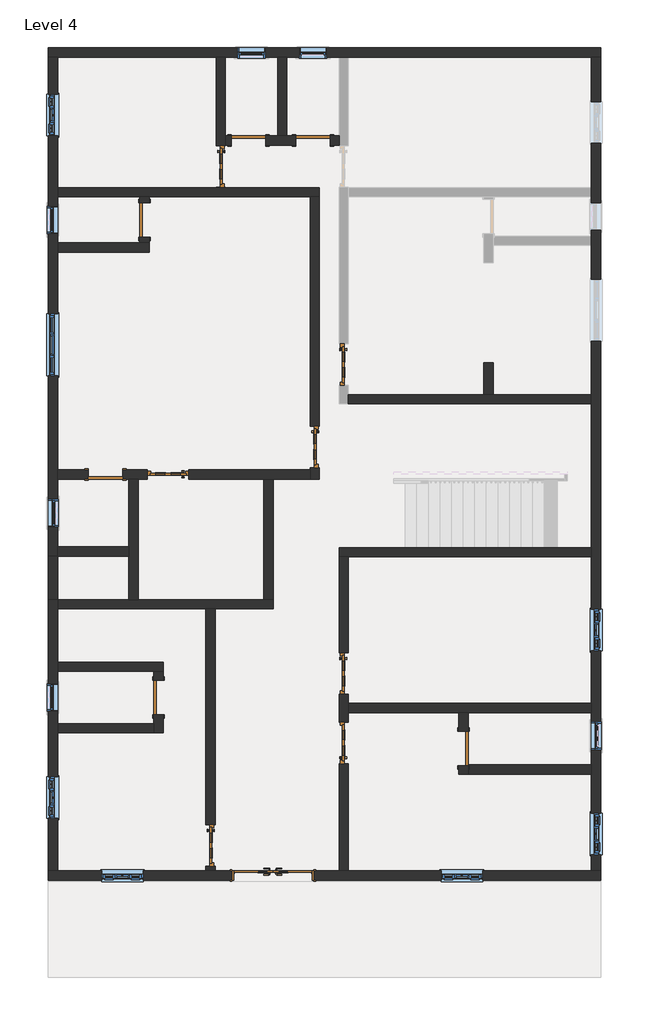
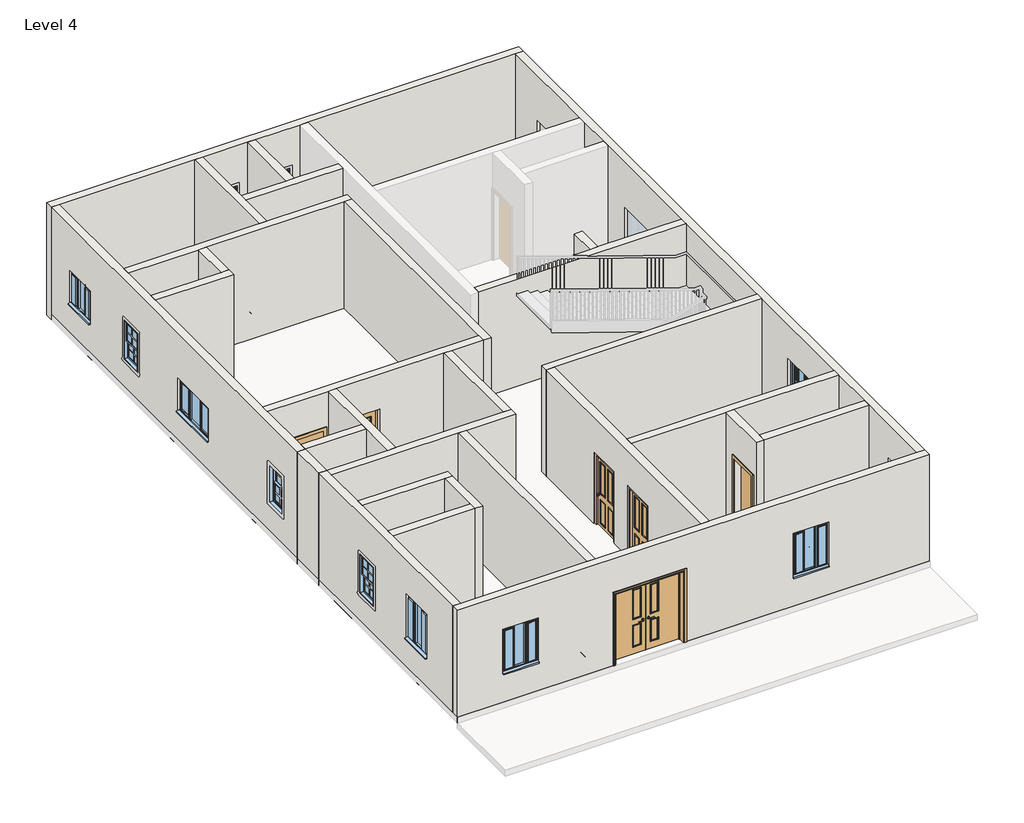
# One storey, part 1 of 3: 29 walls, 14 doors, 13 windows.
"""IFC4 building model written with IfcOpenShell, lengths in millimetres."""

from ifc_helpers import new_model, si_unit, frame, origin, place, context, project, spatial, polyline, outline, extrude, faceted_brep, transform, mapped, element, save
from components import door_2817e3e8, door_51b0c682, doors_intdbl_3_1810x2110mm_301b02ef, doors_intdbl_3_1810x2110mm_13513f6f, door_fadea3f2, door_53b1b562, window_679d2811, windows_tpl_plain_1360x910mm_84993ef1, windows_tpl_w_glazing_cross_bars_910x1210mm_e0b59135, windows_tpl_w_glazing_cross_bars_910x910mm_4aa0f884

model = new_model("IFC4")

# Units and contexts
model_context = context("Model", 3, world=origin())
ifc_project = project(units=[si_unit("LENGTHUNIT", "METRE", prefix="MILLI")], contexts=[model_context])

# Site, building, storey
site = spatial("IfcSite", under=ifc_project)
building = spatial("IfcBuilding", under=site)
storey = spatial("IfcBuildingStorey", under=building, Name="Level 4", Elevation=9144.0)

# Doors
placement = place(None, origin())
door_shape = door_2817e3e8(model_context)
element("IfcDoor", 1, ObjectType="Doors_ExtSgl_2 : 2'x7\"", at=placement, inside=storey, context=model_context, shape_type="MappedRepresentation", body=[
    mapped(door_shape, transform((-2349.4166288, 6357.8803322, 9144.0), x_axis=(0.0, -1.0, 0.0), y_axis=(1.0, 0.0, 0.0), z_axis=(0.0, 0.0, 1.0))),
])
element("IfcDoor", 2, ObjectType="Doors_ExtSgl_2 : 2'x7\"", at=placement, inside=storey, context=model_context, shape_type="MappedRepresentation", body=[
    mapped(door_shape, transform((-286.4451949, 208.0340986, 9144.0), x_axis=(0.0, -1.0, 0.0), y_axis=(1.0, 0.0, 0.0), z_axis=(0.0, 0.0, 1.0))),
])
element("IfcDoor", 3, ObjectType="Doors_ExtSgl_2 : 2'x7\"", at=placement, inside=storey, context=model_context, shape_type="MappedRepresentation", body=[
    mapped(door_shape, transform((348.5548051, -6285.6488489, 9144.0), x_axis=(0.0, 1.0, 0.0), y_axis=(-1.0, 0.0, 0.0), z_axis=(0.0, 0.0, 1.0))),
])
element("IfcDoor", 4, ObjectType="Doors_ExtSgl_2 : 2'x7\"", at=placement, inside=storey, context=model_context, shape_type="MappedRepresentation", body=[
    mapped(door_shape, transform((-2575.1220989, -8536.1734342, 9144.0), x_axis=(0.0, -1.0, 0.0), y_axis=(1.0, 0.0, 0.0), z_axis=(0.0, 0.0, 1.0))),
])
door_2_shape = door_51b0c682(model_context)
element("IfcDoor", 5, ObjectType="Doors_ExtSgl_2 : 2'x7\"", at=placement, inside=storey, context=model_context, shape_type="MappedRepresentation", body=[
    mapped(door_2_shape, transform((348.5548051, -4761.6488489, 9144.0), x_axis=(0.0, -1.0, 0.0), y_axis=(1.0, 0.0, 0.0), z_axis=(0.0, 0.0, 1.0))),
])
element("IfcDoor", 6, ObjectType="Doors_ExtSgl_2 : 2'x7\"", at=placement, inside=storey, context=model_context, shape_type="MappedRepresentation", body=[
    mapped(door_2_shape, transform((-3502.9153286, -401.5659014, 9144.0), x_axis=(-1.0, 0.0, 0.0), y_axis=(0.0, -1.0, 0.0), z_axis=(0.0, 0.0, 1.0))),
])
element("IfcDoor", 7, ObjectType="Doors_ExtSgl_2 : 2'x7\"", at=placement, inside=storey, context=model_context, shape_type="MappedRepresentation", body=[
    mapped(door_2_shape, transform((348.5548051, 2011.4340986, 9144.0), x_axis=(0.0, -1.0, 0.0), y_axis=(1.0, 0.0, 0.0), z_axis=(0.0, 0.0, 1.0))),
])
doors_intdbl_3_1810x2110mm_shape = doors_intdbl_3_1810x2110mm_301b02ef(model_context)
doors_intdbl_3_1810x2110mm_2_shape = doors_intdbl_3_1810x2110mm_13513f6f(model_context)
element("IfcDoor", 8, ObjectType="Doors_IntDbl_3 : 1810x2110mm", at=placement, inside=storey, context=model_context, shape_type="MappedRepresentation", body=[
    mapped(doors_intdbl_3_1810x2110mm_shape, transform((-1203.5220989, -9196.5734342, 9144.0), x_axis=(-1.0, 0.0, 0.0), y_axis=(0.0, -1.0, 0.0), z_axis=(0.0, 0.0, 1.0))),
    mapped(doors_intdbl_3_1810x2110mm_2_shape, transform((-1203.5220989, -9196.5734342, 9144.0), x_axis=(-1.0, 0.0, 0.0), y_axis=(0.0, -1.0, 0.0), z_axis=(0.0, 0.0, 1.0))),
])
door_3_shape = door_fadea3f2(model_context)
element("IfcDoor", 9, ObjectType="Single-Flush : 30\" x 80\"", at=placement, inside=storey, context=model_context, shape_type="MappedRepresentation", body=[
    mapped(door_3_shape, transform((-1739.8166288, 6926.3340986, 9144.0), x_axis=(1.0, 0.0, 0.0), y_axis=(0.0, 1.0, 0.0), z_axis=(0.0, 0.0, 1.0))),
])
element("IfcDoor", 10, ObjectType="Single-Flush : 30\" x 80\"", at=placement, inside=storey, context=model_context, shape_type="MappedRepresentation", body=[
    mapped(door_3_shape, transform((-4874.5153286, -401.5659014, 9144.0), x_axis=(-1.0, 0.0, 0.0), y_axis=(0.0, -1.0, 0.0), z_axis=(0.0, 0.0, 1.0))),
])
door_4_shape = door_53b1b562(model_context)
element("IfcDoor", 11, ObjectType="Single-Flush : 30\" x 80\"", at=placement, inside=storey, context=model_context, shape_type="MappedRepresentation", body=[
    mapped(door_4_shape, transform((-324.5451949, 6926.3340986, 9144.0), x_axis=(-1.0, 0.0, 0.0), y_axis=(0.0, -1.0, 0.0), z_axis=(0.0, 0.0, 1.0))),
])
element("IfcDoor", 12, ObjectType="Single-Flush : 30\" x 80\"", at=placement, inside=storey, context=model_context, shape_type="MappedRepresentation", body=[
    mapped(door_4_shape, transform((-3715.4451949, -5291.0659014, 9144.0), x_axis=(0.0, -1.0, 0.0), y_axis=(1.0, 0.0, 0.0), z_axis=(0.0, 0.0, 1.0))),
])
element("IfcDoor", 13, ObjectType="Single-Flush : 30\" x 80\"", at=placement, inside=storey, context=model_context, shape_type="MappedRepresentation", body=[
    mapped(door_4_shape, transform((2977.4548051, -6412.6488489, 9144.0), x_axis=(0.0, 1.0, 0.0), y_axis=(-1.0, 0.0, 0.0), z_axis=(0.0, 0.0, 1.0))),
])
element("IfcDoor", 14, ObjectType="Single-Flush : 30\" x 80\"", at=placement, inside=storey, context=model_context, shape_type="MappedRepresentation", body=[
    mapped(door_4_shape, transform((-4023.5839448, 5183.1303322, 9144.0), x_axis=(0.0, -1.0, 0.0), y_axis=(1.0, 0.0, 0.0), z_axis=(0.0, 0.0, 1.0))),
])

# Walls
element("IfcWall", 15, ObjectType="Generic - 4.5\" p", at=placement, inside=storey, context=model_context, shape_type="Brep", body=[
    faceted_brep([(-5928.5839448, 5687.8265658, 9144.0), (-4125.1839448, 5687.8265658, 9144.0), (-3921.9839448, 5687.8265658, 9144.0), (-388.0451949, 5687.8265658, 9144.0), (-184.8451949, 5687.8265658, 9144.0), (-184.8451949, 5687.8265658, 12192.0), (-388.0451949, 5687.8265658, 12192.0), (-3921.9839448, 5687.8265658, 12192.0), (-4125.1839448, 5687.8265658, 12192.0), (-5928.5839448, 5687.8265658, 12192.0), (-5928.5839448, 5891.0265658, 9144.0), (-5928.5839448, 5891.0265658, 12192.0), (-2451.0166288, 5891.0265658, 12192.0), (-2247.8166288, 5891.0265658, 12192.0), (-184.8451949, 5891.0265658, 12192.0), (-184.8451949, 5891.0265658, 9144.0), (-2247.8166288, 5891.0265658, 9144.0), (-2451.0166288, 5891.0265658, 9144.0)], [[[0, 1, 2, 3, 4, 5, 6, 7, 8, 9]], [[10, 11, 12, 13, 14, 15, 16, 17]], [[4, 3, 2, 1, 0, 10, 17, 16, 15]], [[0, 9, 11, 10]], [[5, 4, 15, 14]], [[9, 8, 7, 6, 5, 14, 13, 12, 11]]]),
])
element("IfcWall", 16, ObjectType="Generic - 4.5\" p", at=placement, inside=storey, context=model_context, shape_type="Brep", body=[
    faceted_brep([(-388.0451949, -246.9659014, 11254.0), (-388.0451949, -246.9659014, 9144.0), (-388.0451949, -299.9659014, 9144.0), (-388.0451949, -503.1659014, 9144.0), (-388.0451949, -503.1659014, 12192.0), (-388.0451949, -299.9659014, 12192.0), (-388.0451949, 5687.8265658, 12192.0), (-388.0451949, 5687.8265658, 9144.0), (-388.0451949, 663.0340986, 9144.0), (-388.0451949, 663.0340986, 11254.0), (-184.8451949, -503.1659014, 9144.0), (-184.8451949, -246.9659014, 9144.0), (-184.8451949, -246.9659014, 11254.0), (-184.8451949, 663.0340986, 11254.0), (-184.8451949, 663.0340986, 9144.0), (-184.8451949, 5687.8265658, 9144.0), (-184.8451949, 5687.8265658, 12192.0), (-184.8451949, -503.1659014, 12192.0)], [[[0, 1, 2, 3, 4, 5, 6, 7, 8, 9]], [[10, 11, 12, 13, 14, 15, 16, 17]], [[8, 7, 15, 14]], [[3, 2, 1, 11, 10]], [[7, 6, 16, 15]], [[4, 3, 10, 17]], [[14, 13, 9, 8]], [[12, 11, 1, 0]], [[13, 12, 0, 9]], [[6, 5, 4, 17, 16]]]),
])
element("IfcWall", 17, ObjectType="Generic - 4.5\" p", at=placement, inside=storey, context=model_context, shape_type="Brep", body=[
    faceted_brep([(-5255.5153286, -299.9659014, 11176.0), (-5255.5153286, -299.9659014, 9144.0), (-5928.5839448, -299.9659014, 9144.0), (-5928.5839448, -299.9659014, 12192.0), (-388.0451949, -299.9659014, 12192.0), (-388.0451949, -299.9659014, 9144.0), (-3047.9153286, -299.9659014, 9144.0), (-3047.9153286, -299.9659014, 11254.0), (-3957.9153286, -299.9659014, 11254.0), (-3957.9153286, -299.9659014, 9144.0), (-4493.5153286, -299.9659014, 9144.0), (-4493.5153286, -299.9659014, 11176.0), (-5928.5839448, -503.1659014, 9144.0), (-5255.5153286, -503.1659014, 9144.0), (-5255.5153286, -503.1659014, 11176.0), (-4493.5153286, -503.1659014, 11176.0), (-4493.5153286, -503.1659014, 9144.0), (-4366.5153286, -503.1659014, 9144.0), (-4163.3153286, -503.1659014, 9144.0), (-3957.9153286, -503.1659014, 9144.0), (-3957.9153286, -503.1659014, 11254.0), (-3047.9153286, -503.1659014, 11254.0), (-3047.9153286, -503.1659014, 9144.0), (-1404.0451949, -503.1659014, 9144.0), (-1200.8451949, -503.1659014, 9144.0), (-388.0451949, -503.1659014, 9144.0), (-388.0451949, -503.1659014, 12192.0), (-1200.8451949, -503.1659014, 12192.0), (-1404.0451949, -503.1659014, 12192.0), (-4163.3153286, -503.1659014, 12192.0), (-4366.5153286, -503.1659014, 12192.0), (-5928.5839448, -503.1659014, 12192.0)], [[[0, 1, 2, 3, 4, 5, 6, 7, 8, 9, 10, 11]], [[12, 13, 14, 15, 16, 17, 18, 19, 20, 21, 22, 23, 24, 25, 26, 27, 28, 29, 30, 31]], [[6, 5, 25, 24, 23, 22]], [[10, 9, 19, 18, 17, 16]], [[2, 1, 13, 12]], [[5, 4, 26, 25]], [[3, 2, 12, 31]], [[22, 21, 7, 6]], [[20, 19, 9, 8]], [[21, 20, 8, 7]], [[14, 13, 1, 0]], [[15, 14, 0, 11]], [[16, 15, 11, 10]], [[4, 3, 31, 30, 29, 28, 27, 26]]]),
])
element("IfcWall", 18, ObjectType="Generic - 4.5\" p", at=placement, inside=storey, context=model_context, shape_type="Brep", body=[
    faceted_brep([(-4366.5153286, -503.1659014, 9144.0), (-4366.5153286, -1989.0659014, 9144.0), (-4366.5153286, -2192.2659014, 9144.0), (-4366.5153286, -3144.7659014, 9144.0), (-4366.5153286, -3144.7659014, 12192.0), (-4366.5153286, -2192.2659014, 12192.0), (-4366.5153286, -1989.0659014, 12192.0), (-4366.5153286, -503.1659014, 12192.0), (-4163.3153286, -503.1659014, 9144.0), (-4163.3153286, -503.1659014, 12192.0), (-4163.3153286, -3144.7659014, 12192.0), (-4163.3153286, -3144.7659014, 9144.0)], [[[0, 1, 2, 3, 4, 5, 6, 7]], [[8, 9, 10, 11]], [[3, 2, 1, 0, 8, 11]], [[0, 7, 9, 8]], [[4, 3, 11, 10]], [[7, 6, 5, 4, 10, 9]]]),
])
element("IfcWall", 19, ObjectType="Generic - 4.5\" p", at=placement, inside=storey, context=model_context, shape_type="Brep", body=[
    faceted_brep([(-5928.5839448, -3347.9659014, 9144.0), (-2676.7220989, -3347.9659014, 9144.0), (-2473.5220989, -3347.9659014, 9144.0), (-1200.8451949, -3347.9659014, 9144.0), (-1200.8451949, -3347.9659014, 12192.0), (-2473.5220989, -3347.9659014, 12192.0), (-2676.7220989, -3347.9659014, 12192.0), (-5928.5839448, -3347.9659014, 12192.0), (-5928.5839448, -3144.7659014, 9144.0), (-5928.5839448, -3144.7659014, 12192.0), (-4366.5153286, -3144.7659014, 12192.0), (-4163.3153286, -3144.7659014, 12192.0), (-1404.0451949, -3144.7659014, 12192.0), (-1200.8451949, -3144.7659014, 12192.0), (-1200.8451949, -3144.7659014, 9144.0), (-1404.0451949, -3144.7659014, 9144.0), (-4163.3153286, -3144.7659014, 9144.0), (-4366.5153286, -3144.7659014, 9144.0)], [[[0, 1, 2, 3, 4, 5, 6, 7]], [[8, 9, 10, 11, 12, 13, 14, 15, 16, 17]], [[3, 2, 1, 0, 8, 17, 16, 15, 14]], [[0, 7, 9, 8]], [[4, 3, 14, 13]], [[7, 6, 5, 4, 13, 12, 11, 10, 9]]]),
])
element("IfcWall", 20, ObjectType="Generic - 4.5\" p", at=placement, inside=storey, context=model_context, shape_type="SweptSolid", body=[
    extrude(outline(polyline([(-4366.5153286, -2192.2659014), (-5928.5839448, -2192.2659014), (-5928.5839448, -1989.0659014), (-4366.5153286, -1989.0659014), (-4366.5153286, -2192.2659014)])), frame((0.0, 0.0, 9144.0), z_axis=(0.0, 0.0, 1.0), x_axis=(1.0, 0.0, 0.0)), (0.0, 0.0, 1.0), 3048.0),
])
element("IfcWall", 21, ObjectType="Generic - 4.5\" p", at=placement, inside=storey, context=model_context, shape_type="SweptSolid", body=[
    extrude(outline(polyline([(-1404.0451949, -3144.7659014), (-1404.0451949, -503.1659014), (-1200.8451949, -503.1659014), (-1200.8451949, -3144.7659014), (-1404.0451949, -3144.7659014)])), frame((0.0, 0.0, 9144.0), z_axis=(0.0, 0.0, 1.0), x_axis=(1.0, 0.0, 0.0)), (0.0, 0.0, 1.0), 3048.0),
])
element("IfcWall", 22, ObjectType="Generic - 4.5\" p", at=placement, inside=storey, context=model_context, shape_type="Brep", body=[
    faceted_brep([(-5928.5839448, -4719.5659014, 9144.0), (-3817.0451949, -4719.5659014, 9144.0), (-3613.8451949, -4719.5659014, 9144.0), (-3613.8451949, -4719.5659014, 12192.0), (-3817.0451949, -4719.5659014, 12192.0), (-5928.5839448, -4719.5659014, 12192.0), (-5928.5839448, -4516.3659014, 9144.0), (-5928.5839448, -4516.3659014, 12192.0), (-3613.8451949, -4516.3659014, 12192.0), (-3613.8451949, -4516.3659014, 9144.0)], [[[0, 1, 2, 3, 4, 5]], [[6, 7, 8, 9]], [[2, 1, 0, 6, 9]], [[0, 5, 7, 6]], [[3, 2, 9, 8]], [[5, 4, 3, 8, 7]]]),
])
element("IfcWall", 23, ObjectType="Generic - 4.5\" p", at=placement, inside=storey, context=model_context, shape_type="Brep", body=[
    faceted_brep([(-3817.0451949, -5672.0659014, 11176.0), (-3817.0451949, -5672.0659014, 9144.0), (-3817.0451949, -5862.5659014, 9144.0), (-3817.0451949, -6065.7659014, 9144.0), (-3817.0451949, -6065.7659014, 12192.0), (-3817.0451949, -5862.5659014, 12192.0), (-3817.0451949, -4719.5659014, 12192.0), (-3817.0451949, -4719.5659014, 9144.0), (-3817.0451949, -4910.0659014, 9144.0), (-3817.0451949, -4910.0659014, 11176.0), (-3613.8451949, -6065.7659014, 9144.0), (-3613.8451949, -5672.0659014, 9144.0), (-3613.8451949, -5672.0659014, 11176.0), (-3613.8451949, -4910.0659014, 11176.0), (-3613.8451949, -4910.0659014, 9144.0), (-3613.8451949, -4719.5659014, 9144.0), (-3613.8451949, -4719.5659014, 12192.0), (-3613.8451949, -6065.7659014, 12192.0)], [[[0, 1, 2, 3, 4, 5, 6, 7, 8, 9]], [[10, 11, 12, 13, 14, 15, 16, 17]], [[8, 7, 15, 14]], [[3, 2, 1, 11, 10]], [[7, 6, 16, 15]], [[4, 3, 10, 17]], [[12, 11, 1, 0]], [[13, 12, 0, 9]], [[14, 13, 9, 8]], [[6, 5, 4, 17, 16]]]),
])
element("IfcWall", 24, ObjectType="Generic - 4.5\" p", at=placement, inside=storey, context=model_context, shape_type="SweptSolid", body=[
    extrude(outline(polyline([(-5928.5839448, -5862.5659014), (-3817.0451949, -5862.5659014), (-3817.0451949, -6065.7659014), (-5928.5839448, -6065.7659014), (-5928.5839448, -5862.5659014)])), frame((0.0, 0.0, 9144.0), z_axis=(0.0, 0.0, 1.0), x_axis=(1.0, 0.0, 0.0)), (0.0, 0.0, 1.0), 3048.0),
])
element("IfcWall", 25, ObjectType="Generic - 4.5\" p", at=placement, inside=storey, context=model_context, shape_type="SweptSolid", body=[
    extrude(outline(polyline([(-8991.1734342, 11254.0), (-8991.1734342, 9144.0), (-9094.9734342, 9144.0), (-9094.9734342, 12192.0), (-3347.9659014, 12192.0), (-3347.9659014, 9144.0), (-8081.1734342, 9144.0), (-8081.1734342, 11254.0), (-8991.1734342, 11254.0)])), frame((-2676.7220989, 0.0, 0.0), z_axis=(1.0, 0.0, 0.0), x_axis=(0.0, 1.0, 0.0)), (0.0, 0.0, 1.0), 203.2),
])
element("IfcWall", 26, ObjectType="Generic - 4.5\" p", at=placement, inside=storey, context=model_context, shape_type="Brep", body=[
    faceted_brep([(-5928.5839448, 4475.2340986, 9144.0), (-3921.9839448, 4475.2340986, 9144.0), (-3921.9839448, 4475.2340986, 12192.0), (-5928.5839448, 4475.2340986, 12192.0), (-5928.5839448, 4678.4340986, 9144.0), (-5928.5839448, 4678.4340986, 12192.0), (-4125.1839448, 4678.4340986, 12192.0), (-3921.9839448, 4678.4340986, 12192.0), (-3921.9839448, 4678.4340986, 9144.0), (-4125.1839448, 4678.4340986, 9144.0)], [[[0, 1, 2, 3]], [[4, 5, 6, 7, 8, 9]], [[1, 0, 4, 9, 8]], [[0, 3, 5, 4]], [[2, 1, 8, 7]], [[3, 2, 7, 6, 5]]]),
])
element("IfcWall", 27, ObjectType="Generic - 4.5\" p", at=placement, inside=storey, context=model_context, shape_type="SweptSolid", body=[
    extrude(outline(polyline([(4802.1303322, 11176.0), (4802.1303322, 9144.0), (4678.4340986, 9144.0), (4678.4340986, 12192.0), (5687.8265658, 12192.0), (5687.8265658, 9144.0), (5564.1303322, 9144.0), (5564.1303322, 11176.0), (4802.1303322, 11176.0)])), frame((-4125.1839448, 0.0, 0.0), z_axis=(1.0, 0.0, 0.0), x_axis=(0.0, 1.0, 0.0)), (0.0, 0.0, 1.0), 203.2),
])
element("IfcWall", 28, ObjectType="Generic - 4.5\" p", at=placement, inside=storey, context=model_context, shape_type="Brep", body=[
    faceted_brep([(-2451.0166288, 5902.8803322, 11254.0), (-2451.0166288, 5902.8803322, 9144.0), (-2451.0166288, 5891.0265658, 9144.0), (-2451.0166288, 5891.0265658, 12192.0), (-2451.0166288, 8752.5974079, 12192.0), (-2451.0166288, 8752.5974079, 9144.0), (-2451.0166288, 6812.8803322, 9144.0), (-2451.0166288, 6812.8803322, 11254.0), (-2247.8166288, 5891.0265658, 9144.0), (-2247.8166288, 5902.8803322, 9144.0), (-2247.8166288, 5902.8803322, 11254.0), (-2247.8166288, 6812.8803322, 11254.0), (-2247.8166288, 6812.8803322, 9144.0), (-2247.8166288, 6824.7340986, 9144.0), (-2247.8166288, 7027.9340986, 9144.0), (-2247.8166288, 8752.5974079, 9144.0), (-2247.8166288, 8752.5974079, 12192.0), (-2247.8166288, 7027.9340986, 12192.0), (-2247.8166288, 6824.7340986, 12192.0), (-2247.8166288, 5891.0265658, 12192.0)], [[[0, 1, 2, 3, 4, 5, 6, 7]], [[8, 9, 10, 11, 12, 13, 14, 15, 16, 17, 18, 19]], [[6, 5, 15, 14, 13, 12]], [[2, 1, 9, 8]], [[5, 4, 16, 15]], [[3, 2, 8, 19]], [[12, 11, 7, 6]], [[10, 9, 1, 0]], [[11, 10, 0, 7]], [[4, 3, 19, 18, 17, 16]]]),
])
element("IfcWall", 29, ObjectType="Generic - 4.5\" p", at=placement, inside=storey, context=model_context, shape_type="Brep", body=[
    faceted_brep([(-1358.8166288, 6824.7340986, 9144.0), (-705.5451949, 6824.7340986, 9144.0), (-705.5451949, 6824.7340986, 11176.0), (56.4548051, 6824.7340986, 11176.0), (56.4548051, 6824.7340986, 9144.0), (246.9548051, 6824.7340986, 9144.0), (246.9548051, 6824.7340986, 12192.0), (-2247.8166288, 6824.7340986, 12192.0), (-2247.8166288, 6824.7340986, 9144.0), (-2120.8166288, 6824.7340986, 9144.0), (-2120.8166288, 6824.7340986, 11176.0), (-1358.8166288, 6824.7340986, 11176.0), (-705.5451949, 7027.9340986, 11176.0), (-705.5451949, 7027.9340986, 9144.0), (-896.0451949, 7027.9340986, 9144.0), (-1099.2451949, 7027.9340986, 9144.0), (-1358.8166288, 7027.9340986, 9144.0), (-1358.8166288, 7027.9340986, 11176.0), (-2120.8166288, 7027.9340986, 11176.0), (-2120.8166288, 7027.9340986, 9144.0), (-2247.8166288, 7027.9340986, 9144.0), (-2247.8166288, 7027.9340986, 12192.0), (-1099.2451949, 7027.9340986, 12192.0), (-896.0451949, 7027.9340986, 12192.0), (246.9548051, 7027.9340986, 12192.0), (246.9548051, 7027.9340986, 9144.0), (56.4548051, 7027.9340986, 9144.0), (56.4548051, 7027.9340986, 11176.0)], [[[0, 1, 2, 3, 4, 5, 6, 7, 8, 9, 10, 11]], [[12, 13, 14, 15, 16, 17, 18, 19, 20, 21, 22, 23, 24, 25, 26, 27]], [[9, 8, 20, 19]], [[26, 25, 5, 4]], [[16, 15, 14, 13, 1, 0]], [[8, 7, 21, 20]], [[6, 5, 25, 24]], [[17, 16, 0, 11]], [[18, 17, 11, 10]], [[19, 18, 10, 9]], [[2, 1, 13, 12]], [[3, 2, 12, 27]], [[4, 3, 27, 26]], [[7, 6, 24, 23, 22, 21]]]),
])
element("IfcWall", 30, ObjectType="Generic - 4.5\" p", at=placement, inside=storey, context=model_context, shape_type="SweptSolid", body=[
    extrude(outline(polyline([(-1099.2451949, 7027.9340986), (-1099.2451949, 8752.5974079), (-896.0451949, 8752.5974079), (-896.0451949, 7027.9340986), (-1099.2451949, 7027.9340986)])), frame((0.0, 0.0, 9144.0), z_axis=(0.0, 0.0, 1.0), x_axis=(1.0, 0.0, 0.0)), (0.0, 0.0, 1.0), 3048.0),
])
element("IfcWall", 31, ObjectType="Generic - 4.5\" p", at=placement, inside=storey, context=model_context, shape_type="Brep", body=[
    faceted_brep([(450.1548051, 1147.8340986, 9144.0), (5778.5439795, 1147.8340986, 9144.0), (5778.5439795, 1147.8340986, 12192.0), (450.1548051, 1147.8340986, 12192.0), (450.1548051, 1351.0340986, 9144.0), (450.1548051, 1351.0340986, 12192.0), (3421.9548051, 1351.0340986, 12192.0), (3625.1548051, 1351.0340986, 12192.0), (5778.5439795, 1351.0340986, 12192.0), (5778.5439795, 1351.0340986, 9144.0), (3625.1548051, 1351.0340986, 9144.0), (3421.9548051, 1351.0340986, 9144.0)], [[[0, 1, 2, 3]], [[4, 5, 6, 7, 8, 9, 10, 11]], [[1, 0, 4, 11, 10, 9]], [[0, 3, 5, 4]], [[2, 1, 9, 8]], [[3, 2, 8, 7, 6, 5]]]),
])
element("IfcWall", 32, ObjectType="Generic - 4.5\" p", at=placement, inside=storey, context=model_context, shape_type="SweptSolid", body=[
    extrude(outline(polyline([(3625.1548051, 2047.4361958), (3625.1548051, 1351.0340986), (3421.9548051, 1351.0340986), (3421.9548051, 2047.4361958), (3625.1548051, 2047.4361958)])), frame((0.0, 0.0, 9144.0), z_axis=(0.0, 0.0, 1.0), x_axis=(1.0, 0.0, 0.0)), (0.0, 0.0, 1.0), 3048.0),
])
element("IfcWall", 33, ObjectType="Generic - 4.5\" p", at=placement, inside=storey, context=model_context, shape_type="Brep", body=[
    faceted_brep([(5778.5439795, -2004.8977001, 9144.0), (246.9548051, -2004.8977001, 9144.0), (246.9548051, -2004.8977001, 12192.0), (5778.5439795, -2004.8977001, 12192.0), (5778.5439795, -2208.0977001, 9144.0), (5778.5439795, -2208.0977001, 12192.0), (450.1548051, -2208.0977001, 12192.0), (246.9548051, -2208.0977001, 12192.0), (246.9548051, -2208.0977001, 9144.0), (450.1548051, -2208.0977001, 9144.0)], [[[0, 1, 2, 3]], [[4, 5, 6, 7, 8, 9]], [[1, 0, 4, 9, 8]], [[0, 3, 5, 4]], [[2, 1, 8, 7]], [[3, 2, 7, 6, 5]]]),
])
element("IfcWall", 34, ObjectType="Generic - 4.5\" p", at=placement, inside=storey, context=model_context, shape_type="Brep", body=[
    faceted_brep([(246.9548051, -5216.6488489, 9144.0), (246.9548051, -5830.6488489, 9144.0), (246.9548051, -5830.6488489, 11254.0), (246.9548051, -6740.6488489, 11254.0), (246.9548051, -6740.6488489, 9144.0), (246.9548051, -9094.9734342, 9144.0), (246.9548051, -9094.9734342, 12192.0), (246.9548051, -2208.0977001, 12192.0), (246.9548051, -2208.0977001, 9144.0), (246.9548051, -4306.6488489, 9144.0), (246.9548051, -4306.6488489, 11254.0), (246.9548051, -5216.6488489, 11254.0), (450.1548051, -5830.6488489, 11254.0), (450.1548051, -5830.6488489, 9144.0), (450.1548051, -5625.2488489, 9144.0), (450.1548051, -5422.0488489, 9144.0), (450.1548051, -5216.6488489, 9144.0), (450.1548051, -5216.6488489, 11254.0), (450.1548051, -4306.6488489, 11254.0), (450.1548051, -4306.6488489, 9144.0), (450.1548051, -2208.0977001, 9144.0), (450.1548051, -2208.0977001, 12192.0), (450.1548051, -5422.0488489, 12192.0), (450.1548051, -5625.2488489, 12192.0), (450.1548051, -9094.9734342, 12192.0), (450.1548051, -9094.9734342, 9144.0), (450.1548051, -6740.6488489, 9144.0), (450.1548051, -6740.6488489, 11254.0)], [[[0, 1, 2, 3, 4, 5, 6, 7, 8, 9, 10, 11]], [[12, 13, 14, 15, 16, 17, 18, 19, 20, 21, 22, 23, 24, 25, 26, 27]], [[9, 8, 20, 19]], [[26, 25, 5, 4]], [[16, 15, 14, 13, 1, 0]], [[8, 7, 21, 20]], [[6, 5, 25, 24]], [[19, 18, 10, 9]], [[17, 16, 0, 11]], [[18, 17, 11, 10]], [[4, 3, 27, 26]], [[2, 1, 13, 12]], [[3, 2, 12, 27]], [[7, 6, 24, 23, 22, 21]]]),
])
element("IfcWall", 35, ObjectType="Generic - 4.5\" p", at=placement, inside=storey, context=model_context, shape_type="Brep", body=[
    faceted_brep([(450.1548051, -5625.2488489, 9144.0), (2875.8548051, -5625.2488489, 9144.0), (3079.0548051, -5625.2488489, 9144.0), (5778.5439795, -5625.2488489, 9144.0), (5778.5439795, -5625.2488489, 12192.0), (3079.0548051, -5625.2488489, 12192.0), (2875.8548051, -5625.2488489, 12192.0), (450.1548051, -5625.2488489, 12192.0), (450.1548051, -5422.0488489, 9144.0), (450.1548051, -5422.0488489, 12192.0), (5778.5439795, -5422.0488489, 12192.0), (5778.5439795, -5422.0488489, 9144.0)], [[[0, 1, 2, 3, 4, 5, 6, 7]], [[8, 9, 10, 11]], [[3, 2, 1, 0, 8, 11]], [[4, 3, 11, 10]], [[0, 7, 9, 8]], [[7, 6, 5, 4, 10, 9]]]),
])
element("IfcWall", 36, ObjectType="Generic - 4.5\" p", at=placement, inside=storey, context=model_context, shape_type="Brep", body=[
    faceted_brep([(2875.8548051, -5625.2488489, 9144.0), (2875.8548051, -6031.6488489, 9144.0), (2875.8548051, -6031.6488489, 11176.0), (2875.8548051, -6793.6488489, 11176.0), (2875.8548051, -6793.6488489, 9144.0), (2875.8548051, -6971.4488489, 9144.0), (2875.8548051, -6971.4488489, 12192.0), (2875.8548051, -5625.2488489, 12192.0), (3079.0548051, -6031.6488489, 11176.0), (3079.0548051, -6031.6488489, 9144.0), (3079.0548051, -5625.2488489, 9144.0), (3079.0548051, -5625.2488489, 12192.0), (3079.0548051, -6768.2488489, 12192.0), (3079.0548051, -6971.4488489, 12192.0), (3079.0548051, -6971.4488489, 9144.0), (3079.0548051, -6793.6488489, 9144.0), (3079.0548051, -6793.6488489, 11176.0)], [[[0, 1, 2, 3, 4, 5, 6, 7]], [[8, 9, 10, 11, 12, 13, 14, 15, 16]], [[10, 9, 1, 0]], [[15, 14, 5, 4]], [[0, 7, 11, 10]], [[6, 5, 14, 13]], [[2, 1, 9, 8]], [[3, 2, 8, 16]], [[4, 3, 16, 15]], [[7, 6, 13, 12, 11]]]),
])
element("IfcWall", 37, ObjectType="Generic - 4.5\" p", at=placement, inside=storey, context=model_context, shape_type="Brep", body=[
    faceted_brep([(5778.5439795, -6768.2488489, 9144.0), (3079.0548051, -6768.2488489, 9144.0), (3079.0548051, -6768.2488489, 12192.0), (5778.5439795, -6768.2488489, 12192.0), (5778.5439795, -6971.4488489, 9144.0), (5778.5439795, -6971.4488489, 12192.0), (3079.0548051, -6971.4488489, 12192.0), (3079.0548051, -6971.4488489, 9144.0), (3079.0548051, -6793.6488489, 9144.0)], [[[0, 1, 2, 3]], [[4, 5, 6, 7]], [[1, 0, 4, 7, 8]], [[2, 1, 8, 7, 6]], [[0, 3, 5, 4]], [[3, 2, 6, 5]]]),
])
element("IfcWall", 38, ObjectType="Generic - 4.5\" p", at=placement, inside=storey, context=model_context, shape_type="SweptSolid", body=[
    extrude(outline(polyline([(-6131.7839448, -3144.7659014), (-6131.7839448, -2192.2659014), (-5928.5839448, -2192.2659014), (-5928.5839448, -3144.7659014), (-6131.7839448, -3144.7659014)])), frame((0.0, 0.0, 9144.0), z_axis=(0.0, 0.0, 1.0), x_axis=(1.0, 0.0, 0.0)), (0.0, 0.0, 1.0), 3048.0),
])
element("IfcWall", 39, ObjectType="Generic - 9\" w", at=placement, inside=storey, context=model_context, shape_type="Brep", body=[
    faceted_brep([(-6134.0560205, 8752.5974079, 9144.0), (-6131.7839448, 8752.5974079, 9144.0), (-5928.5839448, 8752.5974079, 9144.0), (-2451.0166288, 8752.5974079, 9144.0), (-2247.8166288, 8752.5974079, 9144.0), (-1099.2451949, 8752.5974079, 9144.0), (-896.0451949, 8752.5974079, 9144.0), (246.9548051, 8752.5974079, 9144.0), (450.1548051, 8752.5974079, 9144.0), (5778.5439795, 8752.5974079, 9144.0), (5981.7439795, 8752.5974079, 9144.0), (5981.7439795, 8752.5974079, 12192.0), (5778.5439795, 8752.5974079, 12192.0), (450.1548051, 8752.5974079, 12192.0), (246.9548051, 8752.5974079, 12192.0), (-896.0451949, 8752.5974079, 12192.0), (-1099.2451949, 8752.5974079, 12192.0), (-2247.8166288, 8752.5974079, 12192.0), (-2451.0166288, 8752.5974079, 12192.0), (-5928.5839448, 8752.5974079, 12192.0), (-6131.7839448, 8752.5974079, 12192.0), (-6134.0560205, 8752.5974079, 12192.0), (-1368.7309118, 8752.5974079, 11125.2), (-1368.7309118, 8752.5974079, 10058.4), (-1978.3309118, 8752.5974079, 10058.4), (-1978.3309118, 8752.5974079, 11125.2), (-19.7451949, 8752.5974079, 11125.2), (-19.7451949, 8752.5974079, 10058.4), (-629.3451949, 8752.5974079, 10058.4), (-629.3451949, 8752.5974079, 11125.2), (-6134.0560205, 8955.7974079, 9144.0), (-6134.0560205, 8955.7974079, 12192.0), (5981.7439795, 8955.7974079, 12192.0), (5981.7439795, 8955.7974079, 9144.0), (-1368.7309118, 8955.7974079, 11125.2), (-1978.3309118, 8955.7974079, 11125.2), (-1978.3309118, 8955.7974079, 10058.4), (-1368.7309118, 8955.7974079, 10058.4), (-19.7451949, 8955.7974079, 11125.2), (-629.3451949, 8955.7974079, 11125.2), (-629.3451949, 8955.7974079, 10058.4), (-19.7451949, 8955.7974079, 10058.4)], [[[0, 1, 2, 3, 4, 5, 6, 7, 8, 9, 10, 11, 12, 13, 14, 15, 16, 17, 18, 19, 20, 21], [22, 23, 24, 25], [26, 27, 28, 29]], [[30, 31, 32, 33], [34, 35, 36, 37], [38, 39, 40, 41]], [[10, 9, 8, 7, 6, 5, 4, 3, 2, 1, 0, 30, 33]], [[0, 21, 31, 30]], [[11, 10, 33, 32]], [[23, 22, 34, 37]], [[24, 23, 37, 36]], [[25, 24, 36, 35]], [[22, 25, 35, 34]], [[27, 26, 38, 41]], [[28, 27, 41, 40]], [[29, 28, 40, 39]], [[26, 29, 39, 38]], [[21, 20, 19, 18, 17, 16, 15, 14, 13, 12, 11, 32, 31]]]),
])
element("IfcWall", 40, ObjectType="Generic - 9\" w", at=placement, inside=storey, context=model_context, shape_type="Brep", body=[
    faceted_brep([(5981.7439795, -9094.9734342, 12192.0), (5981.7439795, -9094.9734342, 9144.0), (5778.5439795, -9094.9734342, 9144.0), (450.1548051, -9094.9734342, 9144.0), (246.9548051, -9094.9734342, 9144.0), (-298.5220989, -9094.9734342, 9144.0), (-298.5220989, -9094.9734342, 11254.0), (-2108.5220989, -9094.9734342, 11254.0), (-2108.5220989, -9094.9734342, 9144.0), (-2473.5220989, -9094.9734342, 9144.0), (-2676.7220989, -9094.9734342, 9144.0), (-5928.5839448, -9094.9734342, 9144.0), (-6131.7839448, -9094.9734342, 9144.0), (-6131.7839448, -9094.9734342, 12192.0), (-5928.5839448, -9094.9734342, 12192.0), (-2676.7220989, -9094.9734342, 12192.0), (-2473.5220989, -9094.9734342, 12192.0), (246.9548051, -9094.9734342, 12192.0), (450.1548051, -9094.9734342, 12192.0), (5778.5439795, -9094.9734342, 12192.0), (3394.3548051, -9094.9734342, 11268.4), (2484.3548051, -9094.9734342, 11268.4), (2484.3548051, -9094.9734342, 10058.4), (3394.3548051, -9094.9734342, 10058.4), (-4051.1839448, -9094.9734342, 11268.4), (-4961.1839448, -9094.9734342, 11268.4), (-4961.1839448, -9094.9734342, 10058.4), (-4051.1839448, -9094.9734342, 10058.4), (5981.7439795, -9298.1734342, 9144.0), (5981.7439795, -9298.1734342, 12192.0), (-6131.7839448, -9298.1734342, 12192.0), (-6131.7839448, -9298.1734342, 9144.0), (-2108.5220989, -9298.1734342, 9144.0), (-2108.5220989, -9298.1734342, 11254.0), (-298.5220989, -9298.1734342, 11254.0), (-298.5220989, -9298.1734342, 9144.0), (3394.3548051, -9298.1734342, 11268.4), (3394.3548051, -9298.1734342, 10058.4), (2484.3548051, -9298.1734342, 10058.4), (2484.3548051, -9298.1734342, 11268.4), (-4051.1839448, -9298.1734342, 11268.4), (-4051.1839448, -9298.1734342, 10058.4), (-4961.1839448, -9298.1734342, 10058.4), (-4961.1839448, -9298.1734342, 11268.4)], [[[0, 1, 2, 3, 4, 5, 6, 7, 8, 9, 10, 11, 12, 13, 14, 15, 16, 17, 18, 19], [20, 21, 22, 23], [24, 25, 26, 27]], [[28, 29, 30, 31, 32, 33, 34, 35], [36, 37, 38, 39], [40, 41, 42, 43]], [[1, 28, 35, 5, 4, 3, 2]], [[31, 12, 11, 10, 9, 8, 32]], [[1, 0, 29, 28]], [[13, 12, 31, 30]], [[7, 33, 32, 8]], [[33, 7, 6, 34]], [[34, 6, 5, 35]], [[37, 36, 20, 23]], [[38, 37, 23, 22]], [[39, 38, 22, 21]], [[36, 39, 21, 20]], [[41, 40, 24, 27]], [[42, 41, 27, 26]], [[43, 42, 26, 25]], [[40, 43, 25, 24]], [[0, 19, 18, 17, 16, 15, 14, 13, 30, 29]]]),
])
element("IfcWall", 41, ObjectType="Generic - 9\" w", at=placement, inside=storey, context=model_context, shape_type="Brep", body=[
    faceted_brep([(-5928.5839448, -9094.9734342, 9144.0), (-5928.5839448, -6065.7659014, 9144.0), (-5928.5839448, -5862.5659014, 9144.0), (-5928.5839448, -4719.5659014, 9144.0), (-5928.5839448, -4516.3659014, 9144.0), (-5928.5839448, -3347.9659014, 9144.0), (-5928.5839448, -3144.7659014, 9144.0), (-5928.5839448, -3144.7659014, 12192.0), (-5928.5839448, -3347.9659014, 12192.0), (-5928.5839448, -4516.3659014, 12192.0), (-5928.5839448, -4719.5659014, 12192.0), (-5928.5839448, -5862.5659014, 12192.0), (-5928.5839448, -6065.7659014, 12192.0), (-5928.5839448, -9094.9734342, 12192.0), (-5928.5839448, -7943.1659014, 11268.4), (-5928.5839448, -7033.1659014, 11268.4), (-5928.5839448, -7033.1659014, 10058.4), (-5928.5839448, -7943.1659014, 10058.4), (-5928.5839448, -5595.8659014, 11125.2), (-5928.5839448, -4986.2659014, 11125.2), (-5928.5839448, -4986.2659014, 10058.4), (-5928.5839448, -5595.8659014, 10058.4), (-6131.7839448, -9094.9734342, 9144.0), (-6131.7839448, -9094.9734342, 12192.0), (-6131.7839448, -3144.7659014, 12192.0), (-6131.7839448, -3144.7659014, 9144.0), (-6131.7839448, -7943.1659014, 11268.4), (-6131.7839448, -7943.1659014, 10058.4), (-6131.7839448, -7033.1659014, 10058.4), (-6131.7839448, -7033.1659014, 11268.4), (-6131.7839448, -5595.8659014, 11125.2), (-6131.7839448, -5595.8659014, 10058.4), (-6131.7839448, -4986.2659014, 10058.4), (-6131.7839448, -4986.2659014, 11125.2)], [[[0, 1, 2, 3, 4, 5, 6, 7, 8, 9, 10, 11, 12, 13], [14, 15, 16, 17], [18, 19, 20, 21]], [[22, 23, 24, 25], [26, 27, 28, 29], [30, 31, 32, 33]], [[6, 5, 4, 3, 2, 1, 0, 22, 25]], [[0, 13, 23, 22]], [[7, 6, 25, 24]], [[27, 26, 14, 17]], [[28, 27, 17, 16]], [[29, 28, 16, 15]], [[26, 29, 15, 14]], [[31, 30, 18, 21]], [[32, 31, 21, 20]], [[33, 32, 20, 19]], [[30, 33, 19, 18]], [[13, 12, 11, 10, 9, 8, 7, 24, 23]]]),
])
element("IfcWall", 42, ObjectType="Generic - 9\" w", at=placement, inside=storey, context=model_context, shape_type="Brep", body=[
    faceted_brep([(-5928.5839448, -2192.2659014, 9144.0), (-5928.5839448, -1989.0659014, 9144.0), (-5928.5839448, -503.1659014, 9144.0), (-5928.5839448, -299.9659014, 9144.0), (-5928.5839448, 4475.2340986, 9144.0), (-5928.5839448, 4678.4340986, 9144.0), (-5928.5839448, 5687.8265658, 9144.0), (-5928.5839448, 5891.0265658, 9144.0), (-5928.5839448, 8752.5974079, 9144.0), (-5928.5839448, 8752.5974079, 12192.0), (-5928.5839448, 5891.0265658, 12192.0), (-5928.5839448, 5687.8265658, 12192.0), (-5928.5839448, 4678.4340986, 12192.0), (-5928.5839448, 4475.2340986, 12192.0), (-5928.5839448, -299.9659014, 12192.0), (-5928.5839448, -503.1659014, 12192.0), (-5928.5839448, -1989.0659014, 12192.0), (-5928.5839448, -2192.2659014, 12192.0), (-5928.5839448, 1763.2340986, 10968.4), (-5928.5839448, 3123.2340986, 10968.4), (-5928.5839448, 3123.2340986, 10058.4), (-5928.5839448, 1763.2340986, 10058.4), (-5928.5839448, 7027.5974079, 10968.4), (-5928.5839448, 7937.5974079, 10968.4), (-5928.5839448, 7937.5974079, 10058.4), (-5928.5839448, 7027.5974079, 10058.4), (-5928.5839448, 4878.3303322, 11125.2), (-5928.5839448, 5487.9303322, 11125.2), (-5928.5839448, 5487.9303322, 10058.4), (-5928.5839448, 4878.3303322, 10058.4), (-5928.5839448, -941.3159014, 11125.2), (-5928.5839448, -941.3159014, 10058.4), (-5928.5839448, -1550.9159014, 10058.4), (-5928.5839448, -1550.9159014, 11125.2), (-6131.7839448, -2192.2659014, 9144.0), (-6131.7839448, -2192.2659014, 12192.0), (-6131.7839448, 8752.5974079, 12192.0), (-6131.7839448, 8752.5974079, 9144.0), (-6131.7839448, 1763.2340986, 10968.4), (-6131.7839448, 1763.2340986, 10058.4), (-6131.7839448, 3123.2340986, 10058.4), (-6131.7839448, 3123.2340986, 10968.4), (-6131.7839448, 7027.5974079, 10968.4), (-6131.7839448, 7027.5974079, 10058.4), (-6131.7839448, 7937.5974079, 10058.4), (-6131.7839448, 7937.5974079, 10968.4), (-6131.7839448, 4878.3303322, 11125.2), (-6131.7839448, 4878.3303322, 10058.4), (-6131.7839448, 5487.9303322, 10058.4), (-6131.7839448, 5487.9303322, 11125.2), (-6131.7839448, -941.3159014, 11125.2), (-6131.7839448, -1550.9159014, 11125.2), (-6131.7839448, -1550.9159014, 10058.4), (-6131.7839448, -941.3159014, 10058.4)], [[[0, 1, 2, 3, 4, 5, 6, 7, 8, 9, 10, 11, 12, 13, 14, 15, 16, 17], [18, 19, 20, 21], [22, 23, 24, 25], [26, 27, 28, 29], [30, 31, 32, 33]], [[34, 35, 36, 37], [38, 39, 40, 41], [42, 43, 44, 45], [46, 47, 48, 49], [50, 51, 52, 53]], [[8, 7, 6, 5, 4, 3, 2, 1, 0, 34, 37]], [[9, 8, 37, 36]], [[0, 17, 35, 34]], [[39, 38, 18, 21]], [[40, 39, 21, 20]], [[41, 40, 20, 19]], [[38, 41, 19, 18]], [[43, 42, 22, 25]], [[44, 43, 25, 24]], [[45, 44, 24, 23]], [[42, 45, 23, 22]], [[47, 46, 26, 29]], [[48, 47, 29, 28]], [[49, 48, 28, 27]], [[46, 49, 27, 26]], [[31, 30, 50, 53]], [[32, 31, 53, 52]], [[33, 32, 52, 51]], [[30, 33, 51, 50]], [[17, 16, 15, 14, 13, 12, 11, 10, 9, 36, 35]]]),
])
element("IfcWall", 43, ObjectType="Generic - 9\" w", at=placement, inside=storey, context=model_context, shape_type="Brep", body=[
    faceted_brep([(5778.5439795, 8752.5974079, 9144.0), (5778.5439795, 5891.0265658, 9144.0), (5778.5439795, 5687.8265658, 9144.0), (5778.5439795, 4830.8340986, 9144.0), (5778.5439795, 4627.6340986, 9144.0), (5778.5439795, 1351.0340986, 9144.0), (5778.5439795, 1147.8340986, 9144.0), (5778.5439795, -2004.8977001, 9144.0), (5778.5439795, -2208.0977001, 9144.0), (5778.5439795, -5422.0488489, 9144.0), (5778.5439795, -5625.2488489, 9144.0), (5778.5439795, -6768.2488489, 9144.0), (5778.5439795, -6971.4488489, 9144.0), (5778.5439795, -9094.9734342, 9144.0), (5778.5439795, -9094.9734342, 12192.0), (5778.5439795, -6971.4488489, 12192.0), (5778.5439795, -6768.2488489, 12192.0), (5778.5439795, -5625.2488489, 12192.0), (5778.5439795, -5422.0488489, 12192.0), (5778.5439795, -2208.0977001, 12192.0), (5778.5439795, -2004.8977001, 12192.0), (5778.5439795, 1147.8340986, 12192.0), (5778.5439795, 1351.0340986, 12192.0), (5778.5439795, 4627.6340986, 12192.0), (5778.5439795, 4830.8340986, 12192.0), (5778.5439795, 5687.8265658, 12192.0), (5778.5439795, 5891.0265658, 12192.0), (5778.5439795, 8752.5974079, 12192.0), (5778.5439795, -7827.1734342, 11268.4), (5778.5439795, -8737.1734342, 11268.4), (5778.5439795, -8737.1734342, 10058.4), (5778.5439795, -7827.1734342, 10058.4), (5778.5439795, -3360.0732745, 11268.4), (5778.5439795, -4270.0732745, 11268.4), (5778.5439795, -4270.0732745, 10058.4), (5778.5439795, -3360.0732745, 10058.4), (5778.5439795, 3885.2340986, 10968.4), (5778.5439795, 2525.2340986, 10968.4), (5778.5439795, 2525.2340986, 10058.4), (5778.5439795, 3885.2340986, 10058.4), (5778.5439795, 7776.8119869, 10968.4), (5778.5439795, 6866.8119869, 10968.4), (5778.5439795, 6866.8119869, 10058.4), (5778.5439795, 7776.8119869, 10058.4), (5778.5439795, 4954.5303322, 11125.2), (5778.5439795, 4954.5303322, 10058.4), (5778.5439795, 5564.1303322, 10058.4), (5778.5439795, 5564.1303322, 11125.2), (5778.5439795, -5828.4488489, 11125.2), (5778.5439795, -6438.0488489, 11125.2), (5778.5439795, -6438.0488489, 10058.4), (5778.5439795, -5828.4488489, 10058.4), (5981.7439795, 8752.5974079, 9144.0), (5981.7439795, 8752.5974079, 12192.0), (5981.7439795, -9094.9734342, 12192.0), (5981.7439795, -9094.9734342, 9144.0), (5981.7439795, -7827.1734342, 11268.4), (5981.7439795, -7827.1734342, 10058.4), (5981.7439795, -8737.1734342, 10058.4), (5981.7439795, -8737.1734342, 11268.4), (5981.7439795, -3360.0732745, 11268.4), (5981.7439795, -3360.0732745, 10058.4), (5981.7439795, -4270.0732745, 10058.4), (5981.7439795, -4270.0732745, 11268.4), (5981.7439795, 3885.2340986, 10968.4), (5981.7439795, 3885.2340986, 10058.4), (5981.7439795, 2525.2340986, 10058.4), (5981.7439795, 2525.2340986, 10968.4), (5981.7439795, 7776.8119869, 10968.4), (5981.7439795, 7776.8119869, 10058.4), (5981.7439795, 6866.8119869, 10058.4), (5981.7439795, 6866.8119869, 10968.4), (5981.7439795, 4954.5303322, 11125.2), (5981.7439795, 5564.1303322, 11125.2), (5981.7439795, 5564.1303322, 10058.4), (5981.7439795, 4954.5303322, 10058.4), (5981.7439795, -5828.4488489, 11125.2), (5981.7439795, -5828.4488489, 10058.4), (5981.7439795, -6438.0488489, 10058.4), (5981.7439795, -6438.0488489, 11125.2)], [[[0, 1, 2, 3, 4, 5, 6, 7, 8, 9, 10, 11, 12, 13, 14, 15, 16, 17, 18, 19, 20, 21, 22, 23, 24, 25, 26, 27], [28, 29, 30, 31], [32, 33, 34, 35], [36, 37, 38, 39], [40, 41, 42, 43], [44, 45, 46, 47], [48, 49, 50, 51]], [[52, 53, 54, 55], [56, 57, 58, 59], [60, 61, 62, 63], [64, 65, 66, 67], [68, 69, 70, 71], [72, 73, 74, 75], [76, 77, 78, 79]], [[13, 12, 11, 10, 9, 8, 7, 6, 5, 4, 3, 2, 1, 0, 52, 55]], [[0, 27, 53, 52]], [[14, 13, 55, 54]], [[57, 56, 28, 31]], [[58, 57, 31, 30]], [[59, 58, 30, 29]], [[56, 59, 29, 28]], [[61, 60, 32, 35]], [[62, 61, 35, 34]], [[63, 62, 34, 33]], [[60, 63, 33, 32]], [[65, 64, 36, 39]], [[66, 65, 39, 38]], [[67, 66, 38, 37]], [[64, 67, 37, 36]], [[69, 68, 40, 43]], [[70, 69, 43, 42]], [[71, 70, 42, 41]], [[68, 71, 41, 40]], [[45, 44, 72, 75]], [[46, 45, 75, 74]], [[47, 46, 74, 73]], [[44, 47, 73, 72]], [[77, 76, 48, 51]], [[78, 77, 51, 50]], [[79, 78, 50, 49]], [[76, 79, 49, 48]], [[27, 26, 25, 24, 23, 22, 21, 20, 19, 18, 17, 16, 15, 14, 54, 53]]]),
])

# Windows
window_shape = window_679d2811(model_context)
element("IfcWindow", 44, ObjectType="Window-Double-Hung : 24\" x 42\"", at=placement, inside=storey, context=model_context, shape_type="MappedRepresentation", body=[
    mapped(window_shape, transform((-6030.1839448, 5183.1303322, 9144.0), x_axis=(0.0, 1.0, 0.0), y_axis=(-1.0, 0.0, 0.0), z_axis=(0.0, 0.0, 1.0))),
])
element("IfcWindow", 45, ObjectType="Window-Double-Hung : 24\" x 42\"", at=placement, inside=storey, context=model_context, shape_type="MappedRepresentation", body=[
    mapped(window_shape, transform((-1673.5309118, 8854.1974079, 9144.0), x_axis=(-1.0, 0.0, 0.0), y_axis=(0.0, -1.0, 0.0), z_axis=(0.0, 0.0, 1.0))),
])
element("IfcWindow", 46, ObjectType="Window-Double-Hung : 24\" x 42\"", at=placement, inside=storey, context=model_context, shape_type="MappedRepresentation", body=[
    mapped(window_shape, transform((-324.5451949, 8854.1974079, 9144.0), x_axis=(-1.0, 0.0, 0.0), y_axis=(0.0, -1.0, 0.0), z_axis=(0.0, 0.0, 1.0))),
])
element("IfcWindow", 47, ObjectType="Window-Double-Hung : 24\" x 42\"", at=placement, inside=storey, context=model_context, shape_type="MappedRepresentation", body=[
    mapped(window_shape, transform((5880.1439795, -6133.2488489, 9144.0), x_axis=(0.0, -1.0, 0.0), y_axis=(1.0, 0.0, 0.0), z_axis=(0.0, 0.0, 1.0))),
])
element("IfcWindow", 48, ObjectType="Window-Double-Hung : 24\" x 42\"", at=placement, inside=storey, context=model_context, shape_type="MappedRepresentation", body=[
    mapped(window_shape, transform((-6030.1839448, -5291.0659014, 9144.0), x_axis=(0.0, 1.0, 0.0), y_axis=(-1.0, 0.0, 0.0), z_axis=(0.0, 0.0, 1.0))),
])
element("IfcWindow", 49, ObjectType="Window-Double-Hung : 24\" x 42\"", at=placement, inside=storey, context=model_context, shape_type="MappedRepresentation", body=[
    mapped(window_shape, transform((-6030.1839448, -1246.1159014, 9144.0), x_axis=(0.0, -1.0, 0.0), y_axis=(1.0, 0.0, 0.0), z_axis=(0.0, 0.0, 1.0))),
])
windows_tpl_plain_1360x910mm_shape = windows_tpl_plain_1360x910mm_84993ef1(model_context)
element("IfcWindow", 50, ObjectType="Windows_Tpl_Plain : 1360x910mm", at=placement, inside=storey, context=model_context, shape_type="MappedRepresentation", body=[
    mapped(windows_tpl_plain_1360x910mm_shape, transform((-6021.727377, 2944.9007653, 8858.4), x_axis=(0.0, 1.0, 0.0), y_axis=(-1.0, 0.0, 0.0), z_axis=(0.0, 0.0, 1.0))),
])
windows_tpl_w_glazing_cross_bars_910x1210mm_shape = windows_tpl_w_glazing_cross_bars_910x1210mm_e0b59135(model_context)
element("IfcWindow", 51, ObjectType="Windows_Tpl_w-Glazing_Cross-Bars : 910x1210mm", at=placement, inside=storey, context=model_context, shape_type="MappedRepresentation", body=[
    mapped(windows_tpl_w_glazing_cross_bars_910x1210mm_shape, transform((2512.6881384, -9188.1168663, 9158.4), x_axis=(-1.0, 0.0, 0.0), y_axis=(0.0, -1.0, 0.0), z_axis=(0.0, 0.0, 1.0))),
])
element("IfcWindow", 52, ObjectType="Windows_Tpl_w-Glazing_Cross-Bars : 910x1210mm", at=placement, inside=storey, context=model_context, shape_type="MappedRepresentation", body=[
    mapped(windows_tpl_w_glazing_cross_bars_910x1210mm_shape, transform((-4932.8506115, -9188.1168663, 9158.4), x_axis=(-1.0, 0.0, 0.0), y_axis=(0.0, -1.0, 0.0), z_axis=(0.0, 0.0, 1.0))),
])
element("IfcWindow", 53, ObjectType="Windows_Tpl_w-Glazing_Cross-Bars : 910x1210mm", at=placement, inside=storey, context=model_context, shape_type="MappedRepresentation", body=[
    mapped(windows_tpl_w_glazing_cross_bars_910x1210mm_shape, transform((-6021.727377, -7061.4992347, 9158.4), x_axis=(0.0, 1.0, 0.0), y_axis=(-1.0, 0.0, 0.0), z_axis=(0.0, 0.0, 1.0))),
])
element("IfcWindow", 54, ObjectType="Windows_Tpl_w-Glazing_Cross-Bars : 910x1210mm", at=placement, inside=storey, context=model_context, shape_type="MappedRepresentation", body=[
    mapped(windows_tpl_w_glazing_cross_bars_910x1210mm_shape, transform((5871.6874117, -8708.8401008, 9158.4), x_axis=(0.0, -1.0, 0.0), y_axis=(1.0, 0.0, 0.0), z_axis=(0.0, 0.0, 1.0))),
])
element("IfcWindow", 55, ObjectType="Windows_Tpl_w-Glazing_Cross-Bars : 910x1210mm", at=placement, inside=storey, context=model_context, shape_type="MappedRepresentation", body=[
    mapped(windows_tpl_w_glazing_cross_bars_910x1210mm_shape, transform((5871.6874117, -4241.7399412, 9158.4), x_axis=(0.0, -1.0, 0.0), y_axis=(1.0, 0.0, 0.0), z_axis=(0.0, 0.0, 1.0))),
])
windows_tpl_w_glazing_cross_bars_910x910mm_shape = windows_tpl_w_glazing_cross_bars_910x910mm_4aa0f884(model_context)
element("IfcWindow", 56, ObjectType="Windows_Tpl_w-Glazing_Cross-Bars : 910x910mm", at=placement, inside=storey, context=model_context, shape_type="MappedRepresentation", body=[
    mapped(windows_tpl_w_glazing_cross_bars_910x910mm_shape, transform((-6021.727377, 7909.2640745, 8858.4), x_axis=(0.0, 1.0, 0.0), y_axis=(-1.0, 0.0, 0.0), z_axis=(0.0, 0.0, 1.0))),
])

save(model, "model.ifc")

# Revit data of these elements
# Type "Doors_ExtSgl_2 : 2'x7\""
#   Type Mark = "10"
#   Type Comments = "External Single"
#   Operation = "SingleSwingRight"
#   Construction Type Id = "SGL"
#   Keynote = "L20"
#   Analytic Construction = "Large single-glazed windows"
#   Wrap Layers (Int) from Ext = 0' - 6.98819"
#   Wrap Layers (Ext) from Ext = 0' - 4.03543"
#   Visual Light Transmittance = 0.9
#   Thickness = 0' - 1.73228"
#   Stile Top of Lock rail = 3' - 3.37008"
#   Stile Top Rail = 0' - 5.90551"
#   Stile Shutting = 0' - 4.92126"
#   Stile Muntin Rail = 0' - 4.92126"
#   Stile Lock Rail = 0' - 6.88976"
#   Stile Hanging = 0' - 4.92126"
#   Stile Bottom Rail = 0' - 6.88976"
#   Solar Heat Gain Coefficient = 0.86
#   Rough Width = 2' - 11.82677"
#   Rough Height = 6' - 11.07087"
#   O/A Frame Width = 0' - 2.51969"
#   Heat Transfer Coefficient (U) = 0.979472 BTU/(h·ft²·°F)
#   Handle Z Distance = 3' - 3.37008"
#   Glazing Thickness = 0' - 0.94488"
#   FrameWidth = 0' - 1.65354"
#   FrameOffset - External = 0' - 0.98425"
#   FrameDepth = 0' - 3.50394"
#   Door Panel Width = 2' - 7.77165"
#   Door Panel Thickness = 0' - 1.73228"
#   Door Panel Height = 6' - 6.74016"
#   Cill Thickness = 0' - 2.14567"
#   Cill Projection = 0' - 1.1811"
#   Handle X Distance = 0' - 2.95276"
#   Height = 6' - 11.07087"
#   Structural Tolerance = 0' - 0.25591"
#   Tolerance = 0' - 0.11811"
#   Undercut = 0' - 0.15748"
#   Width = 2' - 11.82677"
#   Cill Extension = 0' - 0.98425"
#   Cavity Closer Width = 0' - 1.9685"
#   Cavity Closer Offset from Ext = 0' - 4.03543"
#   Cavity Closer Depth = 0' - 3.34646"
#   Vis - Ironmongery = yes
#   Vis - Cavity Closers = yes
#   Define Thermal Properties by = 1
#   Function = 1
#   Material Glass = Door - Glazing
#   Material Door = Door - Panel
#   Material Frame = Door - Frame/Mullion
#   Material Ironmongery = Door - Handle
#   Wall Closure = (empty or 0)
# Type "Doors_IntDbl_3 : 1810x2110mm"
#   Type Mark = "11"
#   Type Comments = "Internal Double"
#   Operation = "DoubleDoorSingleSwing"
#   Construction Type Id = "GSP4R"
#   Keynote = "L20"
#   Description = "Internal Double Door"
#   Analytic Construction = "1/8 in Pilkington single glazing"
#   Visual Light Transmittance = 0.9
#   VisionPanel Width = 0' - 7.87402"
#   Thickness = 0' - 1.25984"
#   Stop Thickness = 0' - 0.74803"
#   Stop Depth = 0' - 1.25984"
#   Stile Top Rail = 0' - 8.85827"
#   Stile Shutting = 0' - 4.92126"
#   Stile Lock Rail = 0' - 6.88976"
#   Stile Top of Lock Rail = 3' - 7.30709"
#   Stile Bottom Rail = 1' - 1.77953"
#   Solar Heat Gain Coefficient = 0.78
#   Rough Width = 5' - 11.25984"
#   Rough Height = 6' - 11.07087"
#   Heat Transfer Coefficient (U) = 0.6496 BTU/(h·ft²·°F)
#   Handle Z Distance = 3' - 3.37008"
#   Handle X Distance = 0' - 2.95276"
#   Frame Thickness = 0' - 1.25984"
#   Door Panel Width = 2' - 9.87795"
#   Door Panel Thickness = 0' - 1.25984"
#   Door Panel Height = 6' - 9.10236"
#   Height = 6' - 11.07087"
#   Door Panel Offset = 0' - 0"
#   Structural Tolerance = 0' - 0.31496"
#   Tolerance = 0' - 0.11811"
#   UnderCut = 0' - 0.27559"
#   Width = 5' - 11.25984"
#   Architrave Setback = 0' - 0.19685"
#   Vis - Ironmongery = yes
#   Define Thermal Properties by = 1
#   Material Ironmongery = Door - Handle
#   Material Glass = Door - Glazing
#   Material Frame = Door - Frame/Mullion
#   Material Door = Door - Panel
#   Material Beading = Door - Panel
#   Material Architrave = Door - Architrave
#   Function = (empty or 0)
#   Wall Closure = (empty or 0)
# Type "Single-Flush : 30\" x 80\""
#   Type Mark = "5"
#   Construction Type Id = "MDOOR"
#   Assembly Code = "C1020"
#   Analytic Construction = "Metal"
#   Thickness = 0' - 2"
#   Heat Transfer Coefficient (U) = 0.651978 BTU/(h·ft²·°F)
#   Height = 6' - 8"
#   Trim Projection Ext = 0' - 1"
#   Trim Projection Int = 0' - 1"
#   Trim Width = 0' - 3"
#   Width = 2' - 6"
#   Define Thermal Properties by = 1
#   Define Thermal Properties by = 1
#   Door Material = Door - Panel
#   Frame Material = Door - Frame
#   Visual Light Transmittance = 0
#   Solar Heat Gain Coefficient = 0
#   Function = (empty or 0)
#   Wall Closure = (empty or 0)
# Type "Generic - 4.5\" p"
#   Assembly Code = "B2010"
#   Layers, outside or top first: 0' - 8" no material (function 1)
# Type "Generic - 9\" w"
#   Assembly Code = "B2010"
#   Layers, outside or top first: 0' - 8" no material (function 1)
# Type "Window-Double-Hung : 24\" x 42\""
#   Type Mark = "10"
#   Fire Rating = "0.5h"
#   Construction Type Id = "DG-DR"
#   Assembly Code = "B2020100"
#   Analytic Construction = "Double glazing - domestic"
#   Wall Thickness [instance default] = 0' - 6"
#   Window Inset [instance default] = 0' - 0"
#   Visual Light Transmittance = 0.81
#   Thermal Resistance (R) = 1.8146 (h·ft²·°F)/BTU
#   Solar Heat Gain Coefficient = 0.76
#   Muntin Width = 1' - 6"
#   Muntin Height = 1' - 5 1/8"
#   Interior Wall Closure [instance default] = 0' - 1 1/2"
#   Rough Width = 2' - 0 1/2"
#   Rough Height = 3' - 6 1/2"
#   Frame Extension [instance default] = 0' - 1 1/4"
#   Exterior Wall Closure [instance default] = 0' - 0 1/2"
#   Extension Jamb [instance default] = 0' - 1 1/2"
#   Heat Transfer Coefficient (U) = 0.5511 BTU/(h·ft²·°F)
#   Height = 3' - 6"
#   Width = 2' - 0"
#   Define Thermal Properties by = 1
#   Top Muntin Visibility = yes
#   Indicator Visibility [instance default] = yes
#   Extension Jamb Visibility [instance default] = yes
#   Interior Trim Visibility [instance default] = yes
#   Exterior Trim Visibility [instance default] = yes
#   Define Thermal Properties by = 1
#   Bottom Muntin Visibility = yes
#   Muntin Pattern = Muntin Pattern_2x2 : Muntin Pattern_2x2
#   Interior Trim Material = Wood - Stained
#   Interior Trim = Trim-Window-Interior-Flat : Picture Frame
#   Exterior Trim Material = Clad - White
#   Exterior Trim = Trim-Window-Exterior-Flat : with Sill
#   Glass Panel Material = Glass
#   Exterior Frame Material = Clad - White
#   Interior Frame Material = Wood - Stained
#   Wall Closure = (empty or 0)
# Type "Windows_Tpl_Plain : 1360x910mm"
#   Type Mark = "20"
#   Operation = "TriplePanelVertical"
#   Construction Type Id = "GSP4R"
#   Manufacturer = "Revit"
#   Keynote = "L10"
#   Analytic Construction = "1/8 in Pilkington single glazing"
#   Wrap Layers (Ext) from Ext = 0' - 4.03543"
#   Wrap Layers (Int) from Ext = 0' - 6.98819"
#   Window Board Projection = 0' - 0.98425"
#   Window Board Extension = 0' - 0.98425"
#   Visual Light Transmittance = 0.9
#   Solar Heat Gain Coefficient = 0.78
#   Rough Width = 4' - 5.54331"
#   Rough Height = 2' - 11.82677"
#   Height = 2' - 11.82677"
#   Width = 4' - 5.54331"
#   Heat Transfer Coefficient (U) = 0.6496 BTU/(h·ft²·°F)
#   Glazing Thickness = 0' - 0.94488"
#   FrameOffset - External = 0' - 1.9685"
#   Frame Depth = 0' - 2.55906"
#   Default Head Height = 6' - 11.07087"
#   Cill Depth = 0' - 3.44488"
#   Cavity Closer Width = 0' - 1.9685"
#   Cavity Closer Offset from Ext = 0' - 4.03543"
